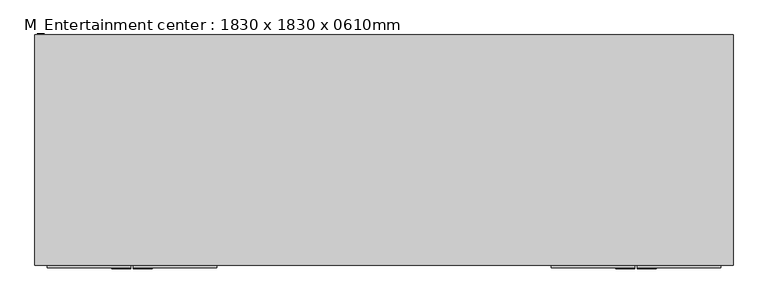
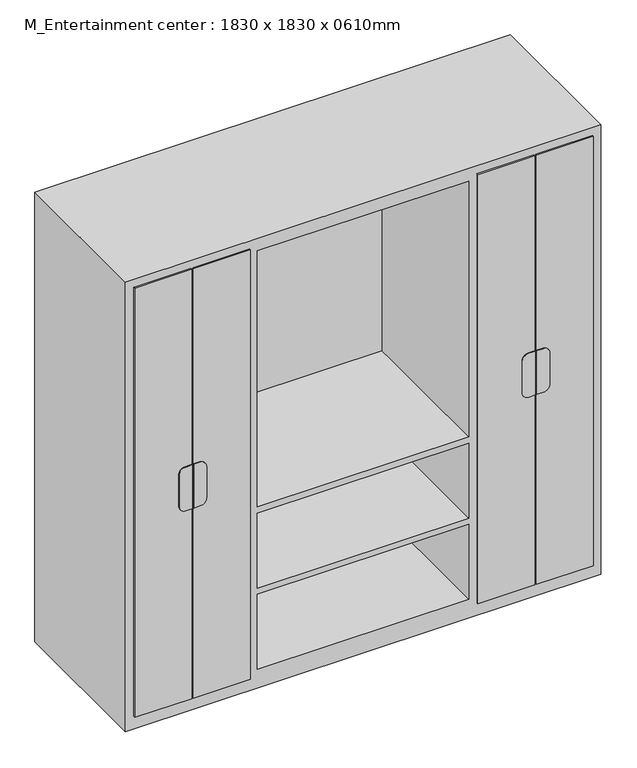
"""IFC4 building model written with IfcOpenShell, lengths in millimetres: furniture geometry, M_Entertainment center : 1830 x 1830 x 0610mm."""

from ifc_helpers import new_model, si_unit, point, frame, frame_2d, origin, place, context, project, spatial, polyline, circle_curve, trimmed, segment, composite_curve, outline, extrude, faceted_brep, source, transform, mapped, element, save


def m_entertainment_center_1830_x_1830_x_0610mm_f77a9b93(model_context):
    return source(origin(), model_context, "Body", "SolidModel", [
        faceted_brep([(915.0, -705.05, 0.0), (915.0, -705.05, 1830.0), (-915.0, -705.05, 1830.0), (-915.0, -705.05, 0.0), (-457.3, -705.05, 1779.2), (-457.3, -705.05, 1385.2), (-864.2, -705.05, 1385.2), (-864.2, -705.05, 1779.2), (-457.3, -705.05, 76.2), (-864.2, -705.05, 76.2), (-864.2, -705.05, 444.8), (-457.3, -705.05, 444.8), (864.2, -705.05, 1385.2), (457.3, -705.05, 1385.2), (457.3, -705.05, 1779.2), (864.2, -705.05, 1779.2), (-406.5, -705.05, 737.2), (-406.5, -705.05, 1779.2), (406.5, -705.05, 1779.2), (406.5, -705.05, 737.2), (406.5, -705.05, 76.2), (-406.5, -705.05, 76.2), (-406.5, -705.05, 381.3), (406.5, -705.05, 381.3), (864.2, -705.05, 76.2), (457.3, -705.05, 76.2), (457.3, -705.05, 444.8), (864.2, -705.05, 444.8), (-864.2, -705.05, 470.2), (-864.2, -705.05, 902.3), (-457.3, -705.05, 902.3), (-457.3, -705.05, 470.2), (-457.3, -705.05, 1359.8), (-457.3, -705.05, 927.7), (-864.2, -705.05, 927.7), (-864.2, -705.05, 1359.8), (457.3, -705.05, 1359.8), (864.2, -705.05, 1359.8), (864.2, -705.05, 927.7), (457.3, -705.05, 927.7), (457.3, -705.05, 902.3), (864.2, -705.05, 902.3), (864.2, -705.05, 470.2), (457.3, -705.05, 470.2), (406.5, -705.05, 406.7), (-406.5, -705.05, 406.7), (-406.5, -705.05, 711.8), (406.5, -705.05, 711.8), (915.0, -101.4, 0.0), (-915.0, -101.4, 0.0), (-915.0, -101.4, 1830.0), (915.0, -101.4, 1830.0), (-457.3, -126.8, 1779.2), (-457.3, -126.8, 1385.2), (-864.2, -126.8, 1385.2), (-864.2, -126.8, 1779.2), (-457.3, -126.8, 76.2), (-864.2, -126.8, 76.2), (-864.2, -126.8, 444.8), (-457.3, -126.8, 444.8), (864.2, -126.8, 1385.2), (457.3, -126.8, 1385.2), (457.3, -126.8, 1779.2), (864.2, -126.8, 1779.2), (-406.5, -126.8, 737.2), (-406.5, -126.8, 1779.2), (406.5, -126.8, 1779.2), (406.5, -126.8, 737.2), (406.5, -126.8, 76.2), (-406.5, -126.8, 76.2), (-406.5, -126.8, 381.3), (406.5, -126.8, 381.3), (864.2, -126.8, 76.2), (457.3, -126.8, 76.2), (457.3, -126.8, 444.8), (864.2, -126.8, 444.8), (-864.2, -126.8, 470.2), (-864.2, -126.8, 902.3), (-457.3, -126.8, 902.3), (-457.3, -126.8, 470.2), (-457.3, -126.8, 1359.8), (-457.3, -126.8, 927.7), (-864.2, -126.8, 927.7), (-864.2, -126.8, 1359.8), (457.3, -126.8, 1359.8), (864.2, -126.8, 1359.8), (864.2, -126.8, 927.7), (457.3, -126.8, 927.7), (457.3, -126.8, 902.3), (864.2, -126.8, 902.3), (864.2, -126.8, 470.2), (457.3, -126.8, 470.2), (406.5, -126.8, 406.7), (-406.5, -126.8, 406.7), (-406.5, -126.8, 711.8), (406.5, -126.8, 711.8)], [[[0, 1, 2, 3], [4, 5, 6, 7], [8, 9, 10, 11], [12, 13, 14, 15], [16, 17, 18, 19], [20, 21, 22, 23], [24, 25, 26, 27], [28, 29, 30, 31], [32, 33, 34, 35], [36, 37, 38, 39], [40, 41, 42, 43], [44, 45, 46, 47]], [[48, 49, 50, 51]], [[1, 0, 48, 51]], [[2, 1, 51, 50]], [[3, 2, 50, 49]], [[0, 3, 49, 48]], [[5, 4, 52, 53]], [[6, 5, 53, 54]], [[7, 6, 54, 55]], [[4, 7, 55, 52]], [[9, 8, 56, 57]], [[10, 9, 57, 58]], [[11, 10, 58, 59]], [[8, 11, 59, 56]], [[13, 12, 60, 61]], [[14, 13, 61, 62]], [[15, 14, 62, 63]], [[12, 15, 63, 60]], [[17, 16, 64, 65]], [[18, 17, 65, 66]], [[19, 18, 66, 67]], [[16, 19, 67, 64]], [[21, 20, 68, 69]], [[22, 21, 69, 70]], [[23, 22, 70, 71]], [[20, 23, 71, 68]], [[25, 24, 72, 73]], [[26, 25, 73, 74]], [[27, 26, 74, 75]], [[24, 27, 75, 72]], [[29, 28, 76, 77]], [[30, 29, 77, 78]], [[31, 30, 78, 79]], [[28, 31, 79, 76]], [[33, 32, 80, 81]], [[34, 33, 81, 82]], [[35, 34, 82, 83]], [[32, 35, 83, 80]], [[37, 36, 84, 85]], [[38, 37, 85, 86]], [[39, 38, 86, 87]], [[36, 39, 87, 84]], [[41, 40, 88, 89]], [[42, 41, 89, 90]], [[43, 42, 90, 91]], [[40, 43, 91, 88]], [[45, 44, 92, 93]], [[46, 45, 93, 94]], [[47, 46, 94, 95]], [[44, 47, 95, 92]], [[53, 52, 55, 54]], [[57, 56, 59, 58]], [[61, 60, 63, 62]], [[65, 64, 67, 66]], [[69, 68, 71, 70]], [[73, 72, 75, 74]], [[77, 76, 79, 78]], [[81, 80, 83, 82]], [[85, 84, 87, 86]], [[89, 88, 91, 90]], [[93, 92, 95, 94]]]),
        extrude(outline(composite_curve([segment(polyline([(1003.9, -633.3486452), (1003.9, -657.575), (826.1, -657.575), (826.1, -633.3486452)]), True, "CONTINUOUS"), segment(trimmed(circle_curve(frame_2d((851.5, -633.3486452)), 25.4), [point((826.1, -633.3486452))], [point((851.5, -607.9486452))], False, "CARTESIAN"), True, "CONTINUOUS"), segment(polyline([(851.5, -607.9486452), (978.5, -607.9486452)]), True, "CONTINUOUS"), segment(trimmed(circle_curve(frame_2d((978.5, -633.3486452)), 25.4), [point((978.5, -607.9486452))], [point((1003.9, -633.3486452))], False, "CARTESIAN"), True, "CONTINUOUS")], self_intersect=False)), frame((0.0, -714.575, 0.0), z_axis=(0.0, 1.0, 0.0), x_axis=(0.0, 0.0, 1.0)), (0.0, 0.0, 1.0), 3.175),
        extrude(outline(composite_curve([segment(trimmed(circle_curve(frame_2d((978.5, -688.53125)), 25.4), [point((1003.9, -688.53125))], [point((978.5, -713.93125))], False, "CARTESIAN"), True, "CONTINUOUS"), segment(polyline([(978.5, -713.93125), (851.5, -713.93125)]), True, "CONTINUOUS"), segment(trimmed(circle_curve(frame_2d((851.5, -688.53125)), 25.4), [point((851.5, -713.93125))], [point((826.1, -688.53125))], False, "CARTESIAN"), True, "CONTINUOUS"), segment(polyline([(826.1, -688.53125), (826.1, -663.925), (1003.9, -663.925), (1003.9, -688.53125)]), True, "CONTINUOUS")], self_intersect=False)), frame((0.0, -714.575, 0.0), z_axis=(0.0, 1.0, 0.0), x_axis=(0.0, 0.0, 1.0)), (0.0, 0.0, 1.0), 3.175),
        extrude(outline(composite_curve([segment(trimmed(circle_curve(frame_2d((978.5, 633.3486452)), 25.4), [point((1003.9, 633.3486452))], [point((978.5, 607.9486452))], False, "CARTESIAN"), True, "CONTINUOUS"), segment(polyline([(978.5, 607.9486452), (851.5, 607.9486452)]), True, "CONTINUOUS"), segment(trimmed(circle_curve(frame_2d((851.5, 633.3486452)), 25.4), [point((851.5, 607.9486452))], [point((826.1, 633.3486452))], False, "CARTESIAN"), True, "CONTINUOUS"), segment(polyline([(826.1, 633.3486452), (826.1, 657.575), (1003.9, 657.575), (1003.9, 633.3486452)]), True, "CONTINUOUS")], self_intersect=False)), frame((0.0, -714.575, 0.0), z_axis=(0.0, 1.0, 0.0), x_axis=(0.0, 0.0, 1.0)), (0.0, 0.0, 1.0), 3.175),
        extrude(outline(composite_curve([segment(polyline([(1003.9, 688.53125), (1003.9, 663.925), (826.1, 663.925), (826.1, 688.53125)]), True, "CONTINUOUS"), segment(trimmed(circle_curve(frame_2d((851.5, 688.53125)), 25.4), [point((826.1, 688.53125))], [point((851.5, 713.93125))], False, "CARTESIAN"), True, "CONTINUOUS"), segment(polyline([(851.5, 713.93125), (978.5, 713.93125)]), True, "CONTINUOUS"), segment(trimmed(circle_curve(frame_2d((978.5, 688.53125)), 25.4), [point((978.5, 713.93125))], [point((1003.9, 688.53125))], False, "CARTESIAN"), True, "CONTINUOUS")], self_intersect=False)), frame((0.0, -714.575, 0.0), z_axis=(0.0, 1.0, 0.0), x_axis=(0.0, 0.0, 1.0)), (0.0, 0.0, 1.0), 3.175),
        extrude(outline(polyline([(-883.25, -705.05), (-663.925, -705.05), (-663.925, -711.4), (-883.25, -711.4), (-883.25, -705.05)])), frame((0.0, 0.0, 50.8), z_axis=(0.0, 0.0, 1.0), x_axis=(1.0, 0.0, 0.0)), (0.0, 0.0, 1.0), 1747.45),
        extrude(outline(polyline([(-657.575, -705.05), (-438.25, -705.05), (-438.25, -711.4), (-657.575, -711.4), (-657.575, -705.05)])), frame((0.0, 0.0, 50.8), z_axis=(0.0, 0.0, 1.0), x_axis=(1.0, 0.0, 0.0)), (0.0, 0.0, 1.0), 1747.45),
        extrude(outline(polyline([(663.925, -705.05), (883.25, -705.05), (883.25, -711.4), (663.925, -711.4), (663.925, -705.05)])), frame((0.0, 0.0, 50.8), z_axis=(0.0, 0.0, 1.0), x_axis=(1.0, 0.0, 0.0)), (0.0, 0.0, 1.0), 1747.45),
        extrude(outline(polyline([(438.25, -705.05), (657.575, -705.05), (657.575, -711.4), (438.25, -711.4), (438.25, -705.05)])), frame((0.0, 0.0, 50.8), z_axis=(0.0, 0.0, 1.0), x_axis=(1.0, 0.0, 0.0)), (0.0, 0.0, 1.0), 1747.45),
    ])


if __name__ == "__main__":
    model = new_model("IFC4")
    model_context = context("Model", 3, world=origin())
    ifc_project = project(units=[si_unit("LENGTHUNIT", "METRE", prefix="MILLI")], contexts=[model_context])
    site = spatial("IfcSite", under=ifc_project)
    building = spatial("IfcBuilding", under=site)
    placement = place(None, origin())
    m_entertainment_center_1830_x_1830_x_0610mm_shape = m_entertainment_center_1830_x_1830_x_0610mm_f77a9b93(model_context)
    element("IfcFurniture", 1, ObjectType="M_Entertainment center : 1830 x 1830 x 0610mm", at=placement, inside=building, context=model_context, shape_type="MappedRepresentation", body=[
        mapped(m_entertainment_center_1830_x_1830_x_0610mm_shape, transform((0.0, 0.0, 0.0), x_axis=(1.0, 0.0, 0.0), y_axis=(0.0, 1.0, 0.0), z_axis=(0.0, 0.0, 1.0))),
    ])
    save(model, "model.ifc")

# Revit data of these elements
# Type "M_Entertainment center : 1830 x 1830 x 0610mm"
#   Center Width = 813 mm
#   Depth = 610 mm
#   Height = 1830 mm
#   Width = 1830 mm
#   Material = Laminate, Ivory, Matte
#   Default Elevation = 0
# Element 1 (IfcFurniture, "M_Entertainment center : 1830 x 1830 x 0610mm")
#   Materials on its faces: "Laminate, Ivory, Matte", "Steel, Chrome Plated", "Glass - Clear, Grey"
# Materials
#   "Laminate, Ivory, Matte": class "Plastic", colour RGB 247 247 229, transparency 0, Description = "Plastic Laminate - Ivory, Matte", Cost = 0
#   "Steel, Chrome Plated": class "Metal", colour RGB 244 244 244, transparency 0, Description = "Chromiuim plated steel", Cost = 0
#   "Glass - Clear, Grey": class "Glass", colour RGB 252 255 255, transparency 0.64
